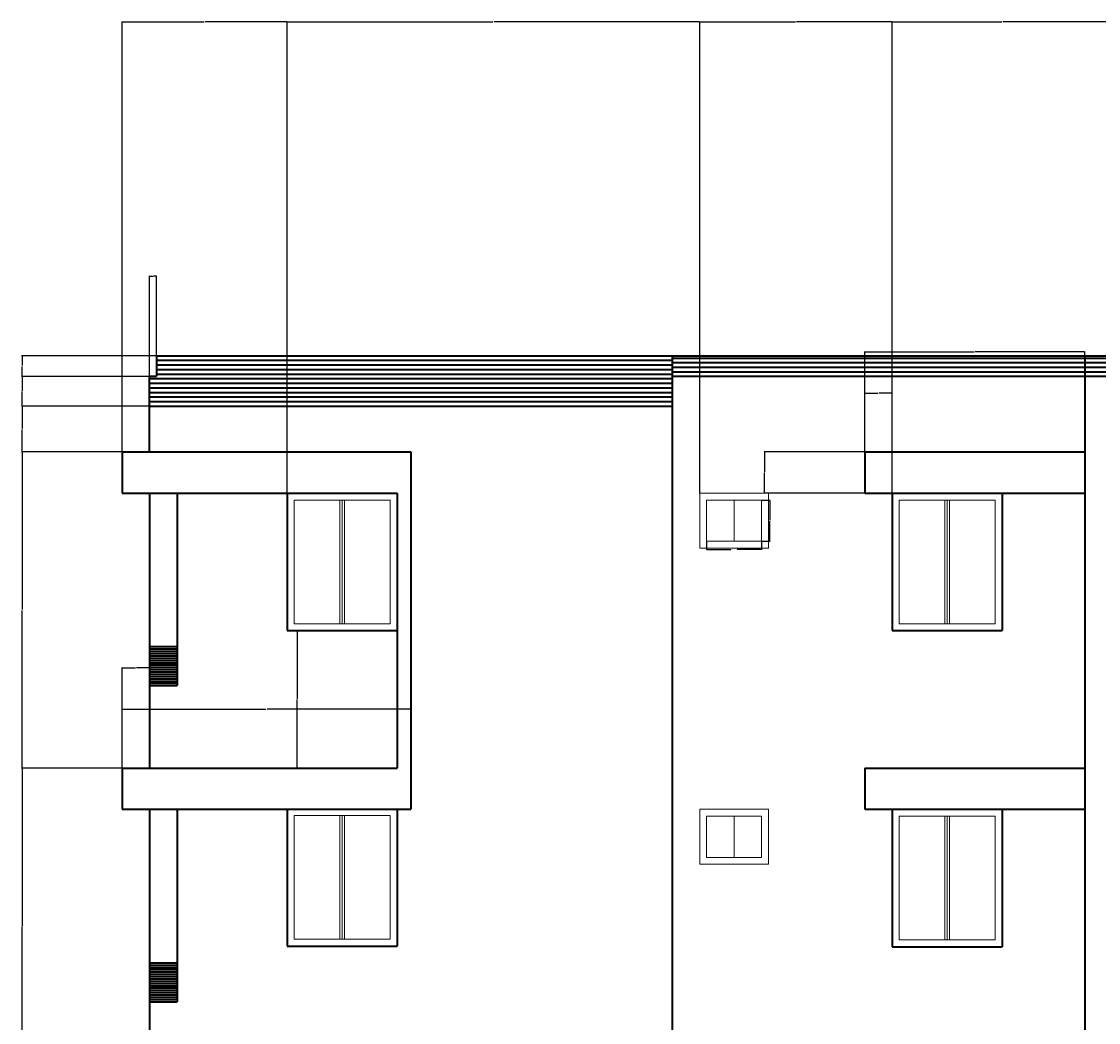
# Model space of a CAD drawing. Units: inches. Extents: x 2136 to 3058, y 322 to 1274.
# Tile 2 of 3: x 2136 to 2606, y 837 to 1274. Entities that reach past the tile are written whole.
import ezdxf

# ---------------------------------------------------------------- set-up
doc = ezdxf.new("R2010")
doc.units = ezdxf.units.IN
for name, color, linetype, lineweight in [('A-ANNO-DIMS', 2, 'Continuous', 18), ('A-ELEV', 7, 'Continuous', 35), ('A-GLAZ', 4, 'Continuous', 18)]:
    doc.layers.add(name, color=color, linetype=linetype, lineweight=lineweight)
doc.styles.get("Standard").update_dxf_attribs({"font": 'arial.ttf'})
doc.dimstyles.get("Standard").update_dxf_attribs({"dimtxt": 0.18, "dimasz": 0.18, "dimexe": 0.18, "dimexo": 0.0625, "dimgap": 0.09, "dimtad": 0, "dimtih": 1, "dimtoh": 1, "dimdec": 4, "dimzin": 0, "dimdsep": 46, "dimtxsty": 'Standard', "dimcen": 0.09, "dimadec": 0, "dimazin": 0, "dimtfac": 1, "dimtdec": 4, "dimtofl": 0, "dimtmove": 0, "dimatfit": 3, "dimfxl": 1, "dimtolj": 1, "dimtzin": 0, "dimarcsym": 0})

# ---------------------------------------------------------------- blocks, each defined once
blk = doc.blocks.new('WIN-SMALL')
for p, q in [((2458.76, 1064.68), (2434.76, 1064.68)), ((2434.76, 1064.68), (2434.76, 1046.68)), ((2446.76, 1064.68), (2446.76, 1046.68)), ((2458.76, 1064.68), (2458.76, 1046.68)), ((2458.76, 1046.68), (2434.76, 1046.68))]:
    blk.add_line(p, q)
blk = doc.blocks.new('WIN-1200')
for p, q in [((2254.76, 650.67), (2254.76, 596.67)), ((2254.76, 650.67), (2296.76, 650.67)), ((2274.76, 596.67), (2274.76, 650.67)), ((2275.76, 596.67), (2275.76, 650.67)), ((2276.76, 596.67), (2276.76, 650.67)), ((2296.76, 650.67), (2296.76, 596.67)), ((2254.76, 596.67), (2296.76, 596.67))]:
    blk.add_line(p, q)
blk = doc.blocks.new('*D4')
at = {"layer": 'A-ANNO-DIMS', "color": 0, "lineweight": -2, "transparency": 16777216}
for p, q in [((2434.76, 1046.62), (2434.76, 1042.9)), ((2458.76, 1046.62), (2458.76, 1042.9)), ((2434.94, 1043.08), (2445.42, 1043.08)), ((2458.58, 1043.08), (2448.1, 1043.08))]:
    blk.add_line(p, q, dxfattribs=at)
at = {"layer": 'A-ANNO-DIMS', "color": 0, "transparency": 16777216}
for points in [[(2434.94, 1043.11), (2434.94, 1043.05), (2434.76, 1043.08)], [(2458.58, 1043.11), (2458.58, 1043.05), (2458.76, 1043.08)]]:
    blk.add_solid(points, dxfattribs=at)
at = {"layer": 'Defpoints', "color": 0, "transparency": 16777216}
for p in [(2434.76, 1046.68), (2458.76, 1046.68), (2458.76, 1043.08)]:
    blk.add_point(p, dxfattribs=at)
at = {"layer": 'A-ANNO-DIMS', "color": 0, "transparency": 16777216, "insert": (2446.76, 1043.08), "char_height": 0.18, "attachment_point": 5}
blk.add_mtext('\\A1;WINDOW W2 24 TYP.', dxfattribs=at)
blk = doc.blocks.new('*D5')
at = {"layer": 'A-ANNO-DIMS', "color": 0, "lineweight": -2, "transparency": 16777216}
for p, q in [((2458.82, 1064.68), (2462.54, 1064.68)), ((2462.36, 1064.5), (2462.36, 1055.87)), ((2462.36, 1046.86), (2462.36, 1055.5)), ((2458.82, 1046.68), (2462.54, 1046.68))]:
    blk.add_line(p, q, dxfattribs=at)
at = {"layer": 'A-ANNO-DIMS', "color": 0, "transparency": 16777216}
for points in [[(2462.33, 1064.5), (2462.39, 1064.5), (2462.36, 1064.68)], [(2462.33, 1046.86), (2462.39, 1046.86), (2462.36, 1046.68)]]:
    blk.add_solid(points, dxfattribs=at)
at = {"layer": 'Defpoints', "color": 0, "transparency": 16777216}
for p in [(2458.76, 1064.68), (2462.36, 1064.68), (2458.76, 1046.68)]:
    blk.add_point(p, dxfattribs=at)
at = {"layer": 'A-ANNO-DIMS', "color": 0, "transparency": 16777216, "insert": (2462.36, 1055.68), "char_height": 0.18, "attachment_point": 5}
blk.add_mtext('\\A1;18 TYP.', dxfattribs=at)
blk = doc.blocks.new('*D17')
at = {"layer": 'A-ANNO-DIMS', "color": 0, "lineweight": -2, "transparency": 16777216}
for p, q in [((2179.7, 947.68), (2135.88, 947.68)), ((2136.06, 947.5), (2136.06, 878.87)), ((2136.06, 809.86), (2136.06, 878.5)), ((2179.7, 809.68), (2135.88, 809.68))]:
    blk.add_line(p, q, dxfattribs=at)
at = {"layer": 'A-ANNO-DIMS', "color": 0, "transparency": 16777216}
for points in [[(2136.03, 947.5), (2136.09, 947.5), (2136.06, 947.68)], [(2136.03, 809.86), (2136.09, 809.86), (2136.06, 809.68)]]:
    blk.add_solid(points, dxfattribs=at)
at = {"layer": 'Defpoints', "color": 0, "transparency": 16777216}
for p in [(2136.06, 947.68), (2179.76, 947.68), (2179.76, 809.68)]:
    blk.add_point(p, dxfattribs=at)
at = {"layer": 'A-ANNO-DIMS', "color": 0, "transparency": 16777216, "insert": (2136.06, 878.68), "char_height": 0.18, "attachment_point": 5}
blk.add_mtext('\\A1;138', dxfattribs=at)
blk = doc.blocks.new('*D18')
at = {"layer": 'A-ANNO-DIMS', "color": 0, "lineweight": -2, "transparency": 16777216}
for p, q in [((2179.7, 1085.68), (2135.88, 1085.68)), ((2136.06, 1085.5), (2136.06, 1016.87)), ((2136.06, 947.86), (2136.06, 1016.5)), ((2179.7, 947.68), (2135.88, 947.68))]:
    blk.add_line(p, q, dxfattribs=at)
at = {"layer": 'A-ANNO-DIMS', "color": 0, "transparency": 16777216}
for points in [[(2136.03, 1085.5), (2136.09, 1085.5), (2136.06, 1085.68)], [(2136.03, 947.86), (2136.09, 947.86), (2136.06, 947.68)]]:
    blk.add_solid(points, dxfattribs=at)
at = {"layer": 'Defpoints', "color": 0, "transparency": 16777216}
for p in [(2136.06, 1085.68), (2179.76, 1085.68), (2179.76, 947.68)]:
    blk.add_point(p, dxfattribs=at)
at = {"layer": 'A-ANNO-DIMS', "color": 0, "transparency": 16777216, "insert": (2136.06, 1016.68), "char_height": 0.18, "attachment_point": 5}
blk.add_mtext('\\A1;138', dxfattribs=at)
blk = doc.blocks.new('*D19')
at = {"layer": 'A-ANNO-DIMS', "color": 0, "lineweight": -2, "transparency": 16777216}
for p, q in [((2191.7, 1105.68), (2135.88, 1105.68)), ((2136.06, 1105.5), (2136.06, 1095.87)), ((2136.06, 1085.86), (2136.06, 1095.5)), ((2179.7, 1085.68), (2135.88, 1085.68))]:
    blk.add_line(p, q, dxfattribs=at)
at = {"layer": 'A-ANNO-DIMS', "color": 0, "transparency": 16777216}
for points in [[(2136.03, 1105.5), (2136.09, 1105.5), (2136.06, 1105.68)], [(2136.03, 1085.86), (2136.09, 1085.86), (2136.06, 1085.68)]]:
    blk.add_solid(points, dxfattribs=at)
at = {"layer": 'Defpoints', "color": 0, "transparency": 16777216}
for p in [(2136.06, 1105.68), (2191.76, 1105.68), (2179.76, 1085.68)]:
    blk.add_point(p, dxfattribs=at)
at = {"layer": 'A-ANNO-DIMS', "color": 0, "transparency": 16777216, "insert": (2136.06, 1095.68), "char_height": 0.18, "attachment_point": 5}
blk.add_mtext('\\A1;20', dxfattribs=at)
blk = doc.blocks.new('*D20')
at = {"layer": 'A-ANNO-DIMS', "color": 0, "lineweight": -2, "transparency": 16777216}
for p, q in [((2191.7, 1118.68), (2135.88, 1118.68)), ((2136.06, 1118.5), (2136.06, 1112.37)), ((2136.06, 1105.86), (2136.06, 1112)), ((2191.7, 1105.68), (2135.88, 1105.68))]:
    blk.add_line(p, q, dxfattribs=at)
at = {"layer": 'A-ANNO-DIMS', "color": 0, "transparency": 16777216}
for points in [[(2136.03, 1118.5), (2136.09, 1118.5), (2136.06, 1118.68)], [(2136.03, 1105.86), (2136.09, 1105.86), (2136.06, 1105.68)]]:
    blk.add_solid(points, dxfattribs=at)
at = {"layer": 'Defpoints', "color": 0, "transparency": 16777216}
for p in [(2136.06, 1118.68), (2191.76, 1118.68), (2191.76, 1105.68)]:
    blk.add_point(p, dxfattribs=at)
at = {"layer": 'A-ANNO-DIMS', "color": 0, "transparency": 16777216, "insert": (2136.06, 1112.18), "char_height": 0.18, "attachment_point": 5}
blk.add_mtext('\\A1;13', dxfattribs=at)
blk = doc.blocks.new('*D21')
at = {"layer": 'A-ANNO-DIMS', "color": 0, "lineweight": -2, "transparency": 16777216}
for p, q in [((2194.7, 1127.68), (2135.88, 1127.68)), ((2136.06, 1127.5), (2136.06, 1123.37)), ((2191.7, 1118.68), (2135.88, 1118.68)), ((2136.06, 1118.86), (2136.06, 1123))]:
    blk.add_line(p, q, dxfattribs=at)
at = {"layer": 'A-ANNO-DIMS', "color": 0, "transparency": 16777216}
for points in [[(2136.03, 1127.5), (2136.09, 1127.5), (2136.06, 1127.68)], [(2136.03, 1118.86), (2136.09, 1118.86), (2136.06, 1118.68)]]:
    blk.add_solid(points, dxfattribs=at)
at = {"layer": 'Defpoints', "color": 0, "transparency": 16777216}
for p in [(2136.06, 1127.68), (2194.76, 1127.68), (2191.76, 1118.68)]:
    blk.add_point(p, dxfattribs=at)
at = {"layer": 'A-ANNO-DIMS', "color": 0, "transparency": 16777216, "insert": (2136.06, 1123.18), "char_height": 0.18, "attachment_point": 5}
blk.add_mtext('\\A1;9', dxfattribs=at)
blk = doc.blocks.new('*D22')
at = {"layer": 'A-ANNO-DIMS', "color": 0, "lineweight": -2, "transparency": 16777216}
for p, q in [((2179.76, 1067.75), (2179.76, 1273.56)), ((2251.76, 1067.75), (2251.76, 1273.56)), ((2179.94, 1273.38), (2215.54, 1273.38)), ((2251.58, 1273.38), (2215.98, 1273.38))]:
    blk.add_line(p, q, dxfattribs=at)
at = {"layer": 'A-ANNO-DIMS', "color": 0, "transparency": 16777216}
for points in [[(2179.94, 1273.41), (2179.94, 1273.35), (2179.76, 1273.38)], [(2251.58, 1273.41), (2251.58, 1273.35), (2251.76, 1273.38)]]:
    blk.add_solid(points, dxfattribs=at)
at = {"layer": 'Defpoints', "color": 0, "transparency": 16777216}
for p in [(2251.76, 1273.38), (2179.76, 1067.68), (2251.76, 1067.68)]:
    blk.add_point(p, dxfattribs=at)
at = {"layer": 'A-ANNO-DIMS', "color": 0, "transparency": 16777216, "insert": (2215.76, 1273.38), "char_height": 0.18, "attachment_point": 5}
blk.add_mtext('\\A1;72', dxfattribs=at)
blk = doc.blocks.new('*D23')
at = {"layer": 'A-ANNO-DIMS', "color": 0, "lineweight": -2, "transparency": 16777216}
for p, q in [((2251.76, 1067.75), (2251.76, 1273.56)), ((2431.76, 1067.75), (2431.76, 1273.56)), ((2251.94, 1273.38), (2341.48, 1273.38)), ((2431.58, 1273.38), (2342.04, 1273.38))]:
    blk.add_line(p, q, dxfattribs=at)
at = {"layer": 'A-ANNO-DIMS', "color": 0, "transparency": 16777216}
for points in [[(2251.94, 1273.41), (2251.94, 1273.35), (2251.76, 1273.38)], [(2431.58, 1273.41), (2431.58, 1273.35), (2431.76, 1273.38)]]:
    blk.add_solid(points, dxfattribs=at)
at = {"layer": 'Defpoints', "color": 0, "transparency": 16777216}
for p in [(2431.76, 1273.38), (2251.76, 1067.68), (2431.76, 1067.68)]:
    blk.add_point(p, dxfattribs=at)
at = {"layer": 'A-ANNO-DIMS', "color": 0, "transparency": 16777216, "insert": (2341.76, 1273.38), "char_height": 0.18, "attachment_point": 5}
blk.add_mtext('\\A1;180', dxfattribs=at)
blk = doc.blocks.new('*D24')
at = {"layer": 'A-ANNO-DIMS', "color": 0, "lineweight": -2, "transparency": 16777216}
for p, q in [((2431.76, 1067.75), (2431.76, 1273.56)), ((2515.76, 1067.75), (2515.76, 1273.56)), ((2431.94, 1273.38), (2473.54, 1273.38)), ((2515.58, 1273.38), (2473.98, 1273.38))]:
    blk.add_line(p, q, dxfattribs=at)
at = {"layer": 'A-ANNO-DIMS', "color": 0, "transparency": 16777216}
for points in [[(2431.94, 1273.41), (2431.94, 1273.35), (2431.76, 1273.38)], [(2515.58, 1273.41), (2515.58, 1273.35), (2515.76, 1273.38)]]:
    blk.add_solid(points, dxfattribs=at)
at = {"layer": 'Defpoints', "color": 0, "transparency": 16777216}
for p in [(2515.76, 1273.38), (2431.76, 1067.68), (2515.76, 1067.68)]:
    blk.add_point(p, dxfattribs=at)
at = {"layer": 'A-ANNO-DIMS', "color": 0, "transparency": 16777216, "insert": (2473.76, 1273.38), "char_height": 0.18, "attachment_point": 5}
blk.add_mtext('\\A1;84', dxfattribs=at)
blk = doc.blocks.new('*D25')
at = {"layer": 'A-ANNO-DIMS', "color": 0, "lineweight": -2, "transparency": 16777216}
for p, q in [((2515.76, 1067.75), (2515.76, 1273.56)), ((2611.76, 1067.75), (2611.76, 1273.56)), ((2515.94, 1273.38), (2563.54, 1273.38)), ((2611.58, 1273.38), (2563.98, 1273.38))]:
    blk.add_line(p, q, dxfattribs=at)
at = {"layer": 'A-ANNO-DIMS', "color": 0, "transparency": 16777216}
for points in [[(2515.94, 1273.41), (2515.94, 1273.35), (2515.76, 1273.38)], [(2611.58, 1273.41), (2611.58, 1273.35), (2611.76, 1273.38)]]:
    blk.add_solid(points, dxfattribs=at)
at = {"layer": 'Defpoints', "color": 0, "transparency": 16777216}
for p in [(2611.76, 1273.38), (2515.76, 1067.68), (2611.76, 1067.68)]:
    blk.add_point(p, dxfattribs=at)
at = {"layer": 'A-ANNO-DIMS', "color": 0, "transparency": 16777216, "insert": (2563.76, 1273.38), "char_height": 0.18, "attachment_point": 5}
blk.add_mtext('\\A1;96', dxfattribs=at)
blk = doc.blocks.new('*D44')
at = {"layer": 'A-ANNO-DIMS', "color": 0, "lineweight": -2, "transparency": 16777216}
for p, q in [((2179.76, 929.75), (2179.76, 973.56)), ((2179.94, 973.38), (2242.48, 973.38)), ((2305.58, 973.38), (2243.04, 973.38)), ((2305.76, 929.75), (2305.76, 973.56))]:
    blk.add_line(p, q, dxfattribs=at)
at = {"layer": 'A-ANNO-DIMS', "color": 0, "transparency": 16777216}
for points in [[(2179.94, 973.41), (2179.94, 973.35), (2179.76, 973.38)], [(2305.58, 973.41), (2305.58, 973.35), (2305.76, 973.38)]]:
    blk.add_solid(points, dxfattribs=at)
at = {"layer": 'Defpoints', "color": 0, "transparency": 16777216}
for p in [(2305.76, 973.38), (2179.76, 929.68), (2305.76, 929.68)]:
    blk.add_point(p, dxfattribs=at)
at = {"layer": 'A-ANNO-DIMS', "color": 0, "transparency": 16777216, "insert": (2242.76, 973.38), "char_height": 0.18, "attachment_point": 5}
blk.add_mtext('\\A1;126', dxfattribs=at)
blk = doc.blocks.new('*D45')
at = {"layer": 'A-ANNO-DIMS', "color": 0, "lineweight": -2, "transparency": 16777216}
for p, q in [((2179.76, 947.75), (2179.76, 991.56)), ((2191.76, 947.75), (2191.76, 991.56)), ((2179.94, 991.38), (2185.55, 991.38)), ((2191.58, 991.38), (2185.97, 991.38))]:
    blk.add_line(p, q, dxfattribs=at)
at = {"layer": 'A-ANNO-DIMS', "color": 0, "transparency": 16777216}
for points in [[(2179.94, 991.41), (2179.94, 991.35), (2179.76, 991.38)], [(2191.58, 991.41), (2191.58, 991.35), (2191.76, 991.38)]]:
    blk.add_solid(points, dxfattribs=at)
at = {"layer": 'Defpoints', "color": 0, "transparency": 16777216}
for p in [(2191.76, 991.38), (2179.76, 947.68), (2191.76, 947.68)]:
    blk.add_point(p, dxfattribs=at)
at = {"layer": 'A-ANNO-DIMS', "color": 0, "transparency": 16777216, "insert": (2185.76, 991.38), "char_height": 0.18, "attachment_point": 5}
blk.add_mtext('\\A1;12', dxfattribs=at)
blk = doc.blocks.new('*D46')
at = {"layer": 'A-ANNO-DIMS', "color": 0, "lineweight": -2, "transparency": 16777216}
for p, q in [((2299.7, 1007.68), (2255.88, 1007.68)), ((2256.06, 1007.5), (2256.06, 977.87)), ((2256.06, 947.86), (2256.06, 977.5)), ((2299.7, 947.68), (2255.88, 947.68))]:
    blk.add_line(p, q, dxfattribs=at)
at = {"layer": 'A-ANNO-DIMS', "color": 0, "transparency": 16777216}
for points in [[(2256.03, 1007.5), (2256.09, 1007.5), (2256.06, 1007.68)], [(2256.03, 947.86), (2256.09, 947.86), (2256.06, 947.68)]]:
    blk.add_solid(points, dxfattribs=at)
at = {"layer": 'Defpoints', "color": 0, "transparency": 16777216}
for p in [(2256.06, 1007.68), (2299.76, 1007.68), (2299.76, 947.68)]:
    blk.add_point(p, dxfattribs=at)
at = {"layer": 'A-ANNO-DIMS', "color": 0, "transparency": 16777216, "insert": (2256.06, 977.68), "char_height": 0.18, "attachment_point": 5}
blk.add_mtext('\\A1;60', dxfattribs=at)
blk = doc.blocks.new('*D47')
at = {"layer": 'A-ANNO-DIMS', "color": 0, "lineweight": -2, "transparency": 16777216}
for p, q in [((2191.76, 1118.75), (2191.76, 1162.56)), ((2191.94, 1162.38), (2193.11, 1162.38)), ((2194.58, 1162.38), (2193.41, 1162.38)), ((2194.76, 1118.75), (2194.76, 1162.56))]:
    blk.add_line(p, q, dxfattribs=at)
at = {"layer": 'A-ANNO-DIMS', "color": 0, "transparency": 16777216}
for points in [[(2191.94, 1162.41), (2191.94, 1162.35), (2191.76, 1162.38)], [(2194.58, 1162.41), (2194.58, 1162.35), (2194.76, 1162.38)]]:
    blk.add_solid(points, dxfattribs=at)
at = {"layer": 'Defpoints', "color": 0, "transparency": 16777216}
for p in [(2194.76, 1162.38), (2191.76, 1118.68), (2194.76, 1118.68)]:
    blk.add_point(p, dxfattribs=at)
at = {"layer": 'A-ANNO-DIMS', "color": 0, "transparency": 16777216, "insert": (2193.26, 1162.38), "char_height": 0.18, "attachment_point": 5}
blk.add_mtext('\\A1;3', dxfattribs=at)
blk = doc.blocks.new('*D48')
at = {"layer": 'A-ANNO-DIMS', "color": 0, "lineweight": -2, "transparency": 16777216}
for p, q in [((2503.76, 1085.75), (2503.76, 1129.56)), ((2503.94, 1129.38), (2551.54, 1129.38)), ((2599.58, 1129.38), (2551.98, 1129.38)), ((2599.76, 1085.75), (2599.76, 1129.56))]:
    blk.add_line(p, q, dxfattribs=at)
at = {"layer": 'A-ANNO-DIMS', "color": 0, "transparency": 16777216}
for points in [[(2503.94, 1129.41), (2503.94, 1129.35), (2503.76, 1129.38)], [(2599.58, 1129.41), (2599.58, 1129.35), (2599.76, 1129.38)]]:
    blk.add_solid(points, dxfattribs=at)
at = {"layer": 'Defpoints', "color": 0, "transparency": 16777216}
for p in [(2599.76, 1129.38), (2503.76, 1085.68), (2599.76, 1085.68)]:
    blk.add_point(p, dxfattribs=at)
at = {"layer": 'A-ANNO-DIMS', "color": 0, "transparency": 16777216, "insert": (2551.76, 1129.38), "char_height": 0.18, "attachment_point": 5}
blk.add_mtext('\\A1;96', dxfattribs=at)
blk = doc.blocks.new('*D49')
at = {"layer": 'A-ANNO-DIMS', "color": 0, "lineweight": -2, "transparency": 16777216}
for p, q in [((2503.76, 1067.75), (2503.76, 1111.56)), ((2503.94, 1111.38), (2509.55, 1111.38)), ((2515.58, 1111.38), (2509.97, 1111.38)), ((2515.76, 1067.75), (2515.76, 1111.56))]:
    blk.add_line(p, q, dxfattribs=at)
at = {"layer": 'A-ANNO-DIMS', "color": 0, "transparency": 16777216}
for points in [[(2503.94, 1111.41), (2503.94, 1111.35), (2503.76, 1111.38)], [(2515.58, 1111.41), (2515.58, 1111.35), (2515.76, 1111.38)]]:
    blk.add_solid(points, dxfattribs=at)
at = {"layer": 'Defpoints', "color": 0, "transparency": 16777216}
for p in [(2515.76, 1111.38), (2503.76, 1067.68), (2515.76, 1067.68)]:
    blk.add_point(p, dxfattribs=at)
at = {"layer": 'A-ANNO-DIMS', "color": 0, "transparency": 16777216, "insert": (2509.76, 1111.38), "char_height": 0.18, "attachment_point": 5}
blk.add_mtext('\\A1;12', dxfattribs=at)
blk = doc.blocks.new('*D50')
at = {"layer": 'A-ANNO-DIMS', "color": 0, "lineweight": -2, "transparency": 16777216}
for p, q in [((2503.7, 1085.68), (2459.88, 1085.68)), ((2460.06, 1085.5), (2460.06, 1076.87)), ((2460.06, 1067.86), (2460.06, 1076.5)), ((2503.7, 1067.68), (2459.88, 1067.68))]:
    blk.add_line(p, q, dxfattribs=at)
at = {"layer": 'A-ANNO-DIMS', "color": 0, "transparency": 16777216}
for points in [[(2460.03, 1085.5), (2460.09, 1085.5), (2460.06, 1085.68)], [(2460.03, 1067.86), (2460.09, 1067.86), (2460.06, 1067.68)]]:
    blk.add_solid(points, dxfattribs=at)
at = {"layer": 'Defpoints', "color": 0, "transparency": 16777216}
for p in [(2460.06, 1085.68), (2503.76, 1085.68), (2503.76, 1067.68)]:
    blk.add_point(p, dxfattribs=at)
at = {"layer": 'A-ANNO-DIMS', "color": 0, "transparency": 16777216, "insert": (2460.06, 1076.68), "char_height": 0.18, "attachment_point": 5}
blk.add_mtext('\\A1;18', dxfattribs=at)

msp = doc.modelspace()

# ---------------------------------------------------------------- linework, layer by layer
at = {"layer": 'A-ELEV'}
for p, q in [((2194.759, 1127.684), (2830.759, 1127.684)), ((2194.759, 1127.684), (2194.759, 1118.684)), ((2194.759, 1125.684), (2419.759, 1125.684)), ((2194.759, 1123.684), (2419.759, 1123.684)), ((2419.759, 1127.684), (2419.759, 395.684)), ((2419.759, 1126.684), (2830.759, 1126.684)), ((2419.759, 1124.684), (2830.759, 1124.684)), ((2599.759, 1127.684), (2599.759, 395.684)), ((2191.759, 1118.684), (2194.759, 1118.684)), ((2191.759, 1085.684), (2191.759, 1118.684)), ((2194.759, 1121.684), (2419.759, 1121.684)), ((2194.759, 1119.684), (2419.759, 1119.684)), ((2419.759, 1122.684), (2830.759, 1122.684)), ((2419.759, 1120.684), (2830.759, 1120.684)), ((2419.759, 1118.684), (2830.759, 1118.684)), ((2191.759, 1117.684), (2419.759, 1117.684)), ((2191.759, 1115.684), (2419.759, 1115.684)), ((2191.759, 1113.684), (2419.759, 1113.684)), ((2191.759, 1111.684), (2419.759, 1111.684)), ((2191.759, 1109.684), (2419.759, 1109.684)), ((2191.759, 1107.684), (2419.759, 1107.684)), ((2191.759, 1105.684), (2419.759, 1105.684)), ((2179.759, 1085.684), (2305.759, 1085.684)), ((2179.759, 1085.684), (2179.759, 1067.684)), ((2305.759, 1085.684), (2305.759, 929.684)), ((2503.759, 1085.684), (2599.759, 1085.684)), ((2503.759, 1085.684), (2503.759, 1067.684)), ((2503.759, 1085.684), (2503.759, 1067.684)), ((2179.759, 1067.684), (2299.759, 1067.684)), ((2191.759, 1067.684), (2191.759, 947.684)), ((2203.759, 1067.684), (2203.759, 983.684)), ((2251.759, 1067.684), (2251.759, 1007.684)), ((2299.759, 1067.684), (2299.759, 947.684)), ((2503.759, 1067.684), (2599.759, 1067.684)), ((2515.759, 1067.684), (2515.759, 1007.684)), ((2563.759, 1067.684), (2563.759, 1007.684)), ((2251.759, 1007.684), (2299.759, 1007.684)), ((2515.759, 1007.684), (2563.759, 1007.684)), ((2191.759, 1000.684), (2203.759, 1000.684)), ((2191.759, 999.684), (2203.759, 999.684)), ((2191.759, 998.684), (2203.759, 998.684)), ((2191.759, 997.684), (2203.759, 997.684)), ((2191.759, 996.684), (2203.759, 996.684)), ((2191.759, 995.684), (2203.759, 995.684)), ((2191.759, 994.684), (2203.759, 994.684)), ((2191.759, 993.684), (2203.759, 993.684)), ((2191.759, 992.684), (2203.759, 992.684)), ((2191.759, 991.684), (2203.759, 991.684)), ((2191.759, 990.684), (2203.759, 990.684)), ((2191.759, 989.684), (2203.759, 989.684)), ((2191.759, 988.684), (2203.759, 988.684)), ((2191.759, 987.684), (2203.759, 987.684)), ((2191.759, 986.684), (2203.759, 986.684)), ((2191.759, 985.684), (2203.759, 985.684)), ((2191.759, 984.684), (2203.759, 984.684)), ((2191.759, 983.684), (2203.759, 983.684)), ((2179.759, 947.684), (2299.759, 947.684)), ((2179.759, 947.684), (2179.759, 929.684)), ((2503.759, 947.684), (2599.759, 947.684)), ((2503.759, 947.684), (2503.759, 929.684)), ((2179.759, 929.684), (2305.759, 929.684)), ((2191.759, 929.684), (2191.759, 809.684)), ((2203.759, 929.684), (2203.759, 845.684)), ((2251.759, 929.931), (2251.759, 869.931)), ((2299.759, 929.684), (2299.759, 869.931)), ((2503.759, 929.684), (2599.759, 929.684)), ((2515.759, 929.684), (2515.759, 869.684)), ((2563.759, 929.684), (2563.759, 869.684)), ((2251.759, 869.931), (2299.759, 869.931)), ((2515.759, 869.684), (2563.759, 869.684)), ((2191.759, 862.684), (2203.759, 862.684)), ((2191.759, 861.684), (2203.759, 861.684)), ((2191.759, 860.684), (2203.759, 860.684)), ((2191.759, 859.684), (2203.759, 859.684)), ((2191.759, 858.684), (2203.759, 858.684)), ((2191.759, 857.684), (2203.759, 857.684)), ((2191.759, 856.684), (2203.759, 856.684)), ((2191.759, 855.684), (2203.759, 855.684)), ((2191.759, 854.684), (2203.759, 854.684)), ((2191.759, 853.684), (2203.759, 853.684)), ((2191.759, 852.684), (2203.759, 852.684)), ((2191.759, 851.684), (2203.759, 851.684)), ((2191.759, 850.684), (2203.759, 850.684)), ((2191.759, 849.684), (2203.759, 849.684)), ((2191.759, 848.684), (2203.759, 848.684)), ((2191.759, 847.684), (2203.759, 847.684)), ((2191.759, 846.684), (2203.759, 846.684)), ((2191.759, 845.684), (2203.759, 845.684))]:
    msp.add_line(p, q, dxfattribs=at)
at = {"layer": 'A-GLAZ'}
for p, q in [((2461.759, 1067.684), (2431.759, 1067.684)), ((2431.759, 1067.684), (2431.759, 1043.684)), ((2461.759, 1067.684), (2461.759, 1043.684)), ((2461.759, 1043.684), (2431.759, 1043.684)), ((2254.759, 926.931), (2254.759, 872.931)), ((2254.759, 926.931), (2296.759, 926.931)), ((2274.759, 872.931), (2274.759, 926.931)), ((2275.759, 872.931), (2275.759, 926.931)), ((2276.759, 872.931), (2276.759, 926.931)), ((2296.759, 926.931), (2296.759, 872.931)), ((2461.759, 929.684), (2431.759, 929.684)), ((2431.759, 929.684), (2431.759, 905.684)), ((2461.759, 929.684), (2461.759, 905.684)), ((2518.759, 926.684), (2518.759, 872.684)), ((2518.759, 926.684), (2560.759, 926.684)), ((2538.759, 926.684), (2538.759, 872.684)), ((2539.759, 926.684), (2539.759, 872.684)), ((2540.759, 926.684), (2540.759, 872.684)), ((2560.759, 926.684), (2560.759, 872.684)), ((2461.759, 905.684), (2431.759, 905.684)), ((2254.759, 872.931), (2296.759, 872.931)), ((2518.759, 872.684), (2560.759, 872.684))]:
    msp.add_line(p, q, dxfattribs=at)

# ---------------------------------------------------------------- block references
at = {"layer": 'A-GLAZ', "rotation": 180}
msp.add_blockref('WIN-1200', (4551.519, 1661.356), dxfattribs=at)
at = {"layer": 'A-GLAZ'}
for name, p in [('WIN-SMALL', (0, 0)), ('WIN-1200', (264, 414.011)), ('WIN-SMALL', (0, -138))]:
    msp.add_blockref(name, p, dxfattribs=at)

# ---------------------------------------------------------------- dimensions: what is measured, and where the dimension line sits
at = {"layer": 'A-ANNO-DIMS'}
for base, p1, p2, picture, middle in [((2251.759, 1273.384), (2179.759, 1067.684), (2251.759, 1067.684), '*D22', (2215.759, 1273.384)), ((2431.759, 1273.384), (2251.759, 1067.684), (2431.759, 1067.684), '*D23', (2341.759, 1273.384)), ((2515.759, 1273.384), (2431.759, 1067.684), (2515.759, 1067.684), '*D24', (2473.759, 1273.384)), ((2611.759, 1273.384), (2515.759, 1067.684), (2611.759, 1067.684), '*D25', (2563.759, 1273.384)), ((2194.759, 1162.384), (2191.759, 1118.684), (2194.759, 1118.684), '*D47', (2193.259, 1162.384)), ((2599.759, 1129.384), (2503.759, 1085.684), (2599.759, 1085.684), '*D48', (2551.759, 1129.384)), ((2515.759, 1111.384), (2503.759, 1067.684), (2515.759, 1067.684), '*D49', (2509.759, 1111.384)), ((2191.759, 991.384), (2179.759, 947.684), (2191.759, 947.684), '*D45', (2185.759, 991.384)), ((2305.759, 973.384), (2179.759, 929.684), (2305.759, 929.684), '*D44', (2242.759, 973.384))]:
    dim = msp.add_linear_dim(base=base, p1=p1, p2=p2, dimstyle='Standard', override={"dimdec": 0, "dimlfac": 1, "dimrnd": 0, "dimzin": 0, "dimdsep": 46, "dimlunit": 2}, dxfattribs=at)
    dim.commit()
    dim.dimension.update_dxf_attribs({"geometry": picture, "text_midpoint": middle})
for base, p1, p2, picture, middle in [((2136.059, 1127.684), (2191.759, 1118.684), (2194.759, 1127.684), '*D21', (2136.059, 1123.184)), ((2136.059, 1118.684), (2191.759, 1105.684), (2191.759, 1118.684), '*D20', (2136.059, 1112.184)), ((2136.059, 1105.684), (2179.759, 1085.684), (2191.759, 1105.684), '*D19', (2136.059, 1095.684)), ((2136.059, 1085.684), (2179.759, 947.684), (2179.759, 1085.684), '*D18', (2136.059, 1016.684)), ((2460.059, 1085.684), (2503.759, 1067.684), (2503.759, 1085.684), '*D50', (2460.059, 1076.684)), ((2256.059, 1007.684), (2299.759, 947.684), (2299.759, 1007.684), '*D46', (2256.059, 977.684)), ((2136.059, 947.684), (2179.759, 809.684), (2179.759, 947.684), '*D17', (2136.059, 878.684))]:
    dim = msp.add_linear_dim(base=base, p1=p1, p2=p2, angle=90, dimstyle='Standard', override={"dimdec": 0, "dimlfac": 1, "dimrnd": 0, "dimzin": 0, "dimdsep": 46, "dimlunit": 2}, dxfattribs=at)
    dim.commit()
    dim.dimension.update_dxf_attribs({"geometry": picture, "text_midpoint": middle})
dim = msp.add_linear_dim(base=(2462.359, 1064.684), p1=(2458.759, 1046.684), p2=(2458.759, 1064.684), angle=90, text='<> TYP.', dimstyle='Standard', override={"dimdec": 0, "dimlfac": 1, "dimrnd": 0, "dimzin": 0, "dimdsep": 46, "dimlunit": 2}, dxfattribs=at)
dim.commit()
dim.dimension.update_dxf_attribs({"geometry": '*D5', "text_midpoint": (2462.359, 1055.684)})
dim = msp.add_linear_dim(base=(2458.759, 1043.084), p1=(2434.759, 1046.684), p2=(2458.759, 1046.684), text='WINDOW W2 <> TYP.', dimstyle='Standard', override={"dimdec": 0, "dimlfac": 1, "dimrnd": 0, "dimzin": 0, "dimdsep": 46, "dimlunit": 2}, dxfattribs=at)
dim.commit()
dim.dimension.update_dxf_attribs({"geometry": '*D4', "text_midpoint": (2446.759, 1043.084)})

doc.saveas('drawing.dxf')
